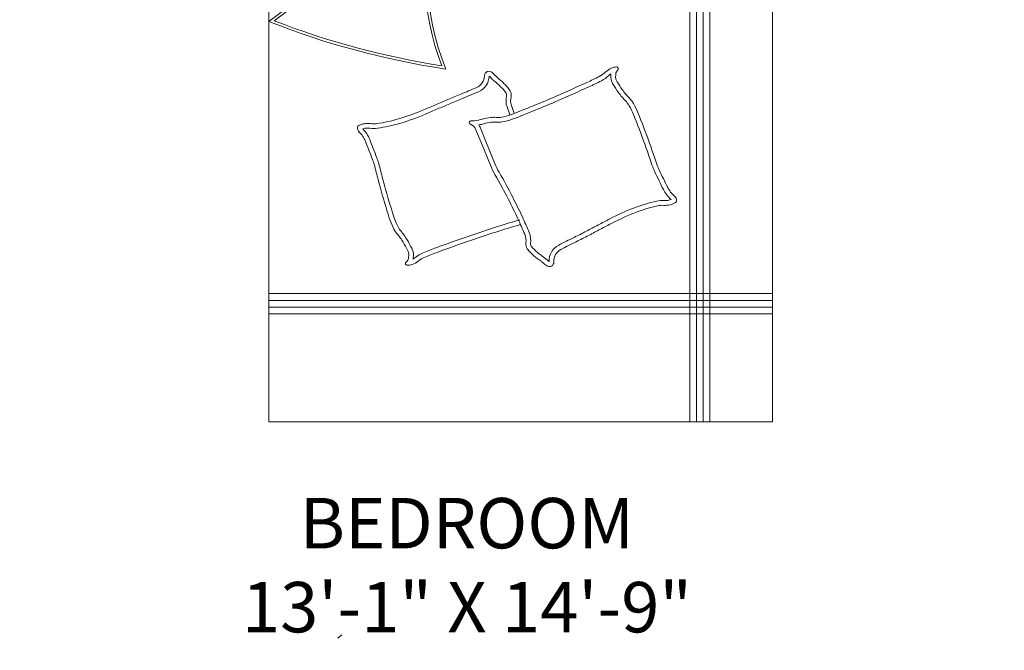
# Model space of a CAD drawing. Units: inches. Extents: x -466983 to 1020, y 324 to 318697.
# Tile 44 of 97: x 491 to 609, y 898 to 973. Entities that reach past the tile are written whole.
import ezdxf

# ---------------------------------------------------------------- set-up
doc = ezdxf.new("R2010")
doc.units = ezdxf.units.IN
doc.header["$MEASUREMENT"] = 0
for name, color, linetype, lineweight in [('A-AREA-IDEN', 7, 'Continuous', 25), ('A-FLOR-PATT', 252, 'Continuous', 13), ('A-FURN', 8, 'Continuous', 18)]:
    doc.layers.add(name, color=color, linetype=linetype, lineweight=lineweight)
doc.styles.get("Standard").update_dxf_attribs({"font": 'arial.ttf'})

# ---------------------------------------------------------------- blocks, each defined once
blk = doc.blocks.new('A$C05F852CF')
for p, q in [((0, 3.0548), (0, 2.6659)), ((0.0306, 3.0783), (0.4692, 3.0783)), ((0.4692, 3.0783), (2.0768, 3.0783)), ((0.52, 3.0783), (0.52, 1.0783)), ((2.02, 3.0783), (2.02, 1.0783)), ((2.0768, 3.0783), (2.5066, 3.0783)), ((0.5, 3.0423), (0.5, 2.6496)), ((0.52, 3.0283), (2.02, 3.0283)), ((2.04, 3.05), (2.04, 2.6642)), ((2.54, 2.6547), (2.54, 3.0393)), ((0.2418, 2.9702), (0.2418, 3.0002)), ((0.5609, 3.0045), (0.5953, 2.9829)), ((0.5609, 3.0045), (0.6121, 2.9725)), ((1.2427, 2.9995), (1.1927, 2.9682)), ((2.2982, 2.9702), (2.2982, 3.0002)), ((0.6121, 2.9725), (0.6546, 2.9682)), ((1.1927, 2.9682), (1.1672, 2.9661)), ((0.1349, 2.8634), (0.1049, 2.8634)), ((0.3487, 2.8634), (0.3787, 2.8634)), ((2.1913, 2.8634), (2.1613, 2.8634)), ((2.4051, 2.8634), (2.4351, 2.8634)), ((0.2418, 2.7265), (0.2418, 2.7565)), ((2.2982, 2.7265), (2.2982, 2.7565)), ((0.5711, 2.6712), (0.6015, 2.7135)), ((0.6015, 2.7135), (0.6164, 2.7178)), ((1.1864, 2.7072), (1.1588, 2.7242)), ((1.2397, 2.6852), (1.1864, 2.7072)), ((1.0379, 2.6608), (0.52, 2.2697)), ((2.02, 2.6608), (1.0379, 2.6608)), ((1.7737, 2.6608), (1.7737, 1.0783)), ((1.7937, 2.6608), (1.7937, 1.0783)), ((1.8137, 2.6608), (1.8137, 1.0783)), ((1.8337, 2.6608), (1.8337, 1.0783)), ((0.0322, 2.6283), (0.4826, 2.6283)), ((2.0707, 2.6283), (2.5056, 2.6283)), ((0.52, 1.4597), (2.02, 1.4597)), ((0.52, 1.4397), (2.02, 1.4397)), ((0.52, 1.4197), (2.02, 1.4197)), ((0.52, 1.3997), (2.02, 1.3997)), ((0.52, 1.0783), (2.02, 1.0783)), ((0.726, 0.4346), (0.7377, 0.4444))]:
    blk.add_line(p, q)
for points in [[(1.3405, 2.9829), (1.306, 3.0045), (1.3573, 2.9725), (1.3998, 2.9682)], [(1.9879, 2.9995), (1.9379, 2.9682), (1.9124, 2.9661)], [(1.3162, 2.6712), (1.3467, 2.7135), (1.3616, 2.7178)], [(1.9848, 2.6852), (1.9315, 2.7072), (1.9039, 2.7242)]]:
    blk.add_lwpolyline(points)
for points in [[(1.0353, 2.1379, -0.173032), (1.022, 2.6388), (0.536, 2.2719, 0.053888)], [(1.7081, 1.7759, 0.101392), (1.7282, 1.7501, -0.223768), (1.7345, 1.736, -0.25558), (1.7315, 1.7308, -0.081563), (1.7151, 1.724, -0.071805), (1.6967, 1.7225, 0.069985), (1.6778, 1.7209, 0.03546), (1.6148, 1.7021, 0.029432), (1.5425, 1.6697, 0.001554), (1.5078, 1.6515, -0.00152), (1.4724, 1.6329, -0.004735), (1.4356, 1.6142, 0.00382), (1.3901, 1.5911, 0.296001), (1.3692, 1.5546, -0.649774), (1.3468, 1.5431, -0.02319), (1.3416, 1.5477, 0.0288), (1.3374, 1.5514, 0.005727), (1.3298, 1.557, -0.004358), (1.3198, 1.5645, -0.027528), (1.3001, 1.5812, -0.046214), (1.29, 1.5928, -0.194121), (1.2856, 1.6105, 0.133719), (1.2823, 1.6363, 0.011505), (1.2622, 1.682, 0.008882), (1.2338, 1.7401, 0.012426), (1.1937, 1.8139, -0.033612), (1.1801, 1.8418), (1.1552, 1.9026), (1.1361, 1.9495, 0.224341), (1.1204, 1.9638, -0.722772), (1.1202, 1.9734, -0.103513), (1.1242, 1.9739, 0.053465), (1.132, 1.9742, 0.030109), (1.1569, 1.9792, -0.031436), (1.1808, 1.984, -0.05324), (1.1971, 1.9844, 0.05518), (1.2128, 1.9849, 0.056271), (1.2402, 1.992, 0.0108), (1.3759, 2.0475, 0.00456), (1.4675, 2.0883, 0.01125), (1.5041, 2.106, 0.069394), (1.5235, 2.1196, -0.079756), (1.5405, 2.1311, -0.106399), (1.5562, 2.1345, -0.328642), (1.5608, 2.1312, -0.299547), (1.5587, 2.124, 0.189917), (1.5536, 2.1141, 0.033518), (1.5531, 2.1029, 0.075627), (1.554, 2.0981, 0.053489), (1.5579, 2.0898, 0.017838), (1.5727, 2.0672, 0.038394), (1.5932, 2.0425, -0.059529), (1.6058, 2.026, -0.035943), (1.6193, 1.9987, -0.011245), (1.6541, 1.9079, -0.006203), (1.6684, 1.8661, 0.010783), (1.6769, 1.8422, 0.019485), (1.6828, 1.8283, 0.005062)], [(1.6953, 1.7695, 0.098587), (1.7181, 1.7399, -0.040378), (1.7118, 1.7379, -0.071805), (1.6975, 1.7367, 0.069985), (1.6747, 1.7349, 0.03546), (1.6097, 1.7154, 0.029432), (1.5359, 1.6824, 0.001554), (1.5012, 1.6641, -0.00152), (1.4658, 1.6456, -0.004735), (1.4293, 1.627, 0.00382), (1.3835, 1.6038, 0.289814), (1.3549, 1.555, -0.018279), (1.3515, 1.5579, 0.0288), (1.3461, 1.5627, 0.005727), (1.3382, 1.5686, -0.004358), (1.3285, 1.5758, -0.027528), (1.31, 1.5916, -0.046214), (1.3016, 1.6012, -0.194121), (1.2997, 1.6085, 0.133719), (1.2955, 1.6417, 0.011505), (1.2752, 1.6881, 0.008882), (1.2465, 1.7466, 0.012426), (1.2061, 1.821, -0.033612), (1.1933, 1.8472), (1.1684, 1.908), (1.1493, 1.9549, 0.051417), (1.1455, 1.962, 0.017208), (1.1606, 1.9654, -0.031436), (1.1827, 1.9698, -0.05324), (1.196, 1.9702, 0.05518), (1.2149, 1.9708, 0.056271), (1.2453, 1.9787, 0.0108), (1.3816, 2.0344, 0.00456), (1.4734, 2.0753, 0.01125), (1.5106, 2.0933, 0.069394), (1.5332, 2.1091, -0.038161), (1.5392, 2.114, 0.029361), (1.5389, 2.1025, 0.075627), (1.5405, 2.0934, 0.053489), (1.5457, 2.0824, 0.017838), (1.5611, 2.0589, 0.038394), (1.583, 2.0326, -0.059529), (1.5935, 2.0187, -0.035943), (1.6061, 1.9933, -0.011245), (1.6406, 1.9031, -0.006203), (1.6549, 1.8617, 0.010783), (1.6635, 1.8371, 0.019485), (1.6699, 1.8222, 0.005062)]]:
    blk.add_lwpolyline(points, format="xyb", close=True)
for points in [[(1.27, 1.665, 0.025626), (1.2575, 1.662, 0.0108), (1.1179, 1.617, 0.00456), (1.0234, 1.5834, 0.01125), (0.9856, 1.5685, 0.069394), (0.9653, 1.5565, -0.079756), (0.9474, 1.5464, -0.106399), (0.9315, 1.5441, -0.328642), (0.9272, 1.5478, -0.299547), (0.9298, 1.5548, 0.189917), (0.9357, 1.5643, 0.033518), (0.9369, 1.5754, 0.075627), (0.9364, 1.5803, 0.053489), (0.9332, 1.5888, 0.017838), (0.9202, 1.6125, 0.038394), (0.9016, 1.6387, -0.059529), (0.8903, 1.6561, -0.035943), (0.8789, 1.6844, -0.011245), (0.8512, 1.7776, -0.006203), (0.8402, 1.8203, 0.010783), (0.8336, 1.8448, 0.019485), (0.8287, 1.8592, 0.005062), (0.8076, 1.9133, 0.101392), (0.7895, 1.9406, -0.223768), (0.7843, 1.9551, -0.25558), (0.7876, 1.9601, -0.081563), (0.8046, 1.9656, -0.071805), (0.823, 1.9657, 0.069985), (0.842, 1.9658, 0.03546), (0.9062, 1.9798, 0.029432), (0.9807, 2.0065, 0.001554), (1.0167, 2.022, -0.00152), (1.0535, 2.0378, -0.004735), (1.0916, 2.0536, 0.00382), (1.1388, 2.0731, 0.296001), (1.1624, 2.108, -0.649774), (1.1856, 2.1178, -0.02319), (1.1904, 2.1128, 0.0288), (1.1944, 2.1088, 0.005727), (1.2015, 2.1025, -0.004358), (1.2108, 2.0944, -0.027528), (1.2292, 2.0762, -0.046214), (1.2384, 2.0638, -0.194121), (1.2414, 2.0458, 0.133719), (1.2427, 2.0199, 0.005779), (1.2507, 1.9961)], [(1.2674, 1.6787, 0.025626), (1.2535, 1.6753, 0.0108), (1.1134, 1.6301, 0.00456), (1.0187, 1.5964, 0.01125), (0.9802, 1.5813, 0.069394), (0.9566, 1.5673, -0.042175), (0.9495, 1.5626, 0.031457), (0.9508, 1.5747, 0.075627), (0.9499, 1.5838, 0.053489), (0.9456, 1.595, 0.017838), (0.9321, 1.6196, 0.038394), (0.9123, 1.6476, -0.059529), (0.9028, 1.6622, -0.035943), (0.8922, 1.6886, -0.011245), (0.8646, 1.7812, -0.006203), (0.8536, 1.8236, 0.010783), (0.8469, 1.8487, 0.019485), (0.8417, 1.8641, 0.005062), (0.8204, 1.9185, 0.100237), (0.7996, 1.9501, -0.044209), (0.8066, 1.9519, -0.071805), (0.8211, 1.952, 0.069985), (0.8439, 1.9521, 0.03546), (0.9101, 1.9665, 0.029432), (0.9862, 1.9937, 0.001554), (1.0222, 2.0093, -0.00152), (1.0589, 2.025, -0.004735), (1.0968, 2.0408, 0.00382), (1.1442, 2.0604, 0.294287), (1.1763, 2.1074, -0.02184), (1.18, 2.1036, 0.0288), (1.1851, 2.0984, 0.005727), (1.1924, 2.092, -0.004358), (1.2016, 2.084, -0.027528), (1.2189, 2.0669, -0.046214), (1.2266, 2.0566, -0.194121), (1.2279, 2.0488, 0.133719), (1.2295, 2.0156, 0.005779), (1.2376, 1.9915, 0.005779)]]:
    blk.add_lwpolyline(points, format="xyb")
for centre, radius in [((0.2418, 2.8634), 0.1369), ((2.2982, 2.8634), 0.1369), ((0.2418, 2.8634), 0.1069), ((2.2982, 2.8634), 0.1069)]:
    blk.add_circle(centre, radius)
for centre, radius, start, end in [((1.7308, 2.407), 0.7379, 159.8846, 202.2194), ((1.4058, 4.5145), 2.4132, 248.4641, 261.4655)]:
    blk.add_arc(centre, radius, start, end)
for points in [[(0, 3.0548), (0, 3.0677), (0.0177, 3.0783), (0.0306, 3.0783)], [(0.5, 3.0423), (0.5, 3.0581), (0.485, 3.0783), (0.4692, 3.0783)], [(2.04, 3.05), (2.04, 3.0655), (2.0613, 3.0783), (2.0768, 3.0783)], [(2.5066, 3.0783), (2.5237, 3.0783), (2.54, 3.0564), (2.54, 3.0393)], [(0.0322, 2.6283), (0.0157, 2.6283), (0, 2.6494), (0, 2.6659)], [(0.5, 2.6496), (0.5, 2.6405), (0.4918, 2.6283), (0.4826, 2.6283)], [(2.04, 2.6642), (2.04, 2.6485), (2.055, 2.6283), (2.0707, 2.6283)], [(2.5056, 2.6283), (2.5201, 2.6283), (2.54, 2.6403), (2.54, 2.6547)]]:
    blk.add_open_spline(points, degree=3)
for points, knots in [([(0.5609, 3.0045), (0.565, 2.9818), (0.5836, 2.9366), (0.5776, 2.889), (0.5689, 2.8351), (0.5832, 2.7709), (0.5808, 2.7088), (0.5744, 2.6927), (0.5693, 2.6651), (0.5803, 2.6793), (0.5989, 2.6876), (0.7172, 2.6598), (0.8681, 2.7029), (1.0484, 2.6781), (1.0324, 2.6731), (1.1431, 2.7116), (1.202, 2.6757), (1.2459, 2.6867), (1.2222, 2.695), (1.2359, 2.7251), (1.2468, 2.781), (1.2288, 2.8492), (1.2515, 2.925), (1.2279, 2.9609), (1.2471, 3.0058), (1.2098, 2.9902), (1.1177, 3.0095), (0.956, 3.0159), (0.9532, 2.9758), (0.7999, 3.021), (0.7569, 3.0151), (0.5986, 2.9869), (0.561, 3.0049)], [16.816032, 16.816032, 16.816032, 16.816032, 79.038845, 88.513895, 147.565266, 227.196862, 259.685448, 283.955301, 296.511304, 302.432558, 320.230942, 354.322559, 575.279549, 734.72356, 845.740421, 943.033103, 1029.533967, 1032.845074, 1043.313584, 1065.311534, 1104.921835, 1208.53002, 1248.510714, 1303.102727, 1321.01326, 1329.647833, 1389.371624, 1571.817644, 1750.274161, 1823.189073, 1967.937033, 2020.912329, 2020.912329, 2020.912329, 2020.912329]), ([(1.306, 3.0045), (1.3102, 2.9818), (1.3287, 2.9366), (1.3228, 2.889), (1.314, 2.8351), (1.3284, 2.7709), (1.3259, 2.7088), (1.3196, 2.6927), (1.3144, 2.6651), (1.3254, 2.6793), (1.3441, 2.6876), (1.4624, 2.6598), (1.6132, 2.7029), (1.6436, 2.6781), (1.7775, 2.6731), (1.8882, 2.7116), (1.9472, 2.6757), (1.9911, 2.6867), (1.9673, 2.695), (1.981, 2.7251), (1.992, 2.781), (1.974, 2.8492), (1.9967, 2.925), (1.9731, 2.9609), (1.9922, 3.0058), (1.9549, 2.9902), (1.8628, 3.0095), (1.7011, 3.0159), (1.5483, 2.9758), (1.5451, 3.021), (1.5021, 3.0151), (1.3437, 2.9869), (1.3062, 3.0049)], [16.816032, 16.816032, 16.816032, 16.816032, 79.038845, 88.513895, 147.565266, 227.196862, 259.685448, 283.955301, 296.511304, 302.432558, 320.230942, 354.322559, 575.279549, 734.72356, 845.740421, 943.033103, 1029.533967, 1032.845074, 1043.313584, 1065.311534, 1104.921835, 1208.53002, 1248.510714, 1303.102727, 1321.01326, 1329.647833, 1389.371624, 1571.817644, 1750.274161, 1823.189073, 1967.937033, 2020.912329, 2020.912329, 2020.912329, 2020.912329]), ([(1.186, 2.943), (1.1557, 2.9456), (1.1387, 2.9502), (1.0976, 2.9551), (1.0776, 2.9567), (1.0342, 2.9582), (1.0123, 2.957), (0.991, 2.9533), (0.9902, 2.9517), (0.962, 2.9403), (0.9371, 2.935), (0.8851, 2.9413), (0.8522, 2.9513), (0.8033, 2.9629), (0.7938, 2.964), (0.755, 2.9608), (0.7319, 2.9572), (0.6794, 2.9481), (0.658, 2.9434), (0.631, 2.9418)], [1364.380335, 1364.380335, 1364.380335, 1364.380335, 1423.60231, 1423.60231, 1482.824284, 1482.824284, 1566.205036, 1566.205036, 1649.585789, 1649.585789, 1732.966542, 1732.966542, 1816.347295, 1816.347295, 1899.728048, 1899.728048, 1960.499853, 1960.499853, 1990.525565, 1990.525565, 1990.525565, 1990.525565]), ([(0.631, 2.9418), (0.6332, 2.9288), (0.633, 2.9104), (0.6308, 2.893), (0.6298, 2.8865), (0.628, 2.8726), (0.6273, 2.866), (0.6257, 2.8474), (0.6257, 2.8375), (0.629, 2.8013), (0.6345, 2.7696), (0.6337, 2.7333)], [67.285362, 67.285362, 67.285362, 67.285362, 87.399558, 87.399558, 107.513754, 107.513754, 127.62795, 127.62795, 167.856341, 167.856341, 238.127268, 238.127268, 238.127268, 238.127268]), ([(1.1845, 2.7412), (1.189, 2.7552), (1.1894, 2.765), (1.1874, 2.7998), (1.1843, 2.8219), (1.1844, 2.8664), (1.1882, 2.8901), (1.192, 2.9105), (1.1922, 2.9144), (1.1921, 2.9158), (1.1908, 2.9212), (1.1875, 2.9351), (1.1867, 2.9388), (1.186, 2.943)], [1072.516901, 1072.516901, 1072.516901, 1072.516901, 1129.100964, 1129.100964, 1185.685027, 1185.685027, 1226.035089, 1226.035089, 1249.281274, 1249.281274, 1272.52746, 1272.52746, 1279.689275, 1279.689275, 1279.689275, 1279.689275]), ([(1.3759, 2.942), (1.3781, 2.929), (1.378, 2.9106), (1.3757, 2.893), (1.3748, 2.8866), (1.373, 2.8727), (1.3722, 2.8661), (1.3706, 2.8475), (1.3707, 2.8375), (1.3739, 2.8012), (1.3795, 2.7694), (1.3787, 2.7331)], [67.156228, 67.156228, 67.156228, 67.156228, 87.297212, 87.297212, 107.438196, 107.438196, 127.57918, 127.57918, 167.861148, 167.861148, 238.25357, 238.25357, 238.25357, 238.25357]), ([(1.5104, 2.9621), (1.4964, 2.9606), (1.4732, 2.9568), (1.4226, 2.948), (1.4017, 2.9435), (1.3759, 2.942)], [1904.3965, 1904.3965, 1904.3965, 1904.3965, 1961.927876, 1961.927876, 1990.619445, 1990.619445, 1990.619445, 1990.619445]), ([(1.9314, 2.9432), (1.8997, 2.9459), (1.8822, 2.9507), (1.8387, 2.9557), (1.8168, 2.9572), (1.7515, 2.9587), (1.7088, 2.9551), (1.6403, 2.9447), (1.6154, 2.9402), (1.5795, 2.937), (1.5675, 2.9361), (1.5394, 2.9412), (1.5201, 2.9507), (1.5104, 2.9621)], [1364.265661, 1364.265661, 1364.265661, 1364.265661, 1426.240795, 1426.240795, 1488.215928, 1488.215928, 1612.166195, 1612.166195, 1689.92864, 1689.92864, 1733.064362, 1733.064362, 1768.978829, 1768.978829, 1768.978829, 1768.978829]), ([(1.9299, 2.7409), (1.9344, 2.755), (1.9348, 2.7648), (1.9328, 2.7996), (1.9297, 2.8217), (1.9298, 2.8662), (1.9336, 2.8899), (1.9374, 2.9105), (1.9376, 2.9144), (1.9375, 2.9159), (1.9362, 2.9214), (1.9329, 2.9353), (1.9321, 2.939), (1.9314, 2.9432)], [1072.238498, 1072.238498, 1072.238498, 1072.238498, 1128.864869, 1128.864869, 1185.491239, 1185.491239, 1225.989553, 1225.989553, 1249.326401, 1249.326401, 1272.66325, 1272.66325, 1279.788508, 1279.788508, 1279.788508, 1279.788508]), ([(0.6337, 2.7333), (0.6515, 2.7301), (0.6627, 2.7284), (0.6898, 2.7263), (0.7032, 2.726), (0.7436, 2.727), (0.7707, 2.73), (0.8409, 2.7383), (0.8881, 2.7432), (0.9755, 2.7406), (1.0125, 2.7357), (1.0356, 2.7309), (1.0369, 2.7307), (1.0381, 2.7304)], [345.4047, 345.4047, 345.4047, 345.4047, 383.386056, 383.386056, 421.367413, 421.367413, 497.330126, 497.330126, 611.561469, 611.561469, 725.792813, 725.792813, 732.434768, 732.434768, 732.434768, 732.434768]), ([(1.0381, 2.7304), (1.0497, 2.7345), (1.0742, 2.7435), (1.1251, 2.7504), (1.1528, 2.749), (1.1769, 2.7432), (1.1809, 2.7421), (1.1845, 2.7412)], [843.64503, 843.64503, 843.64503, 843.64503, 911.27572, 911.27572, 959.088062, 959.088062, 969.47998, 969.47998, 969.47998, 969.47998]), ([(1.3787, 2.7331), (1.3984, 2.7296), (1.4106, 2.7278), (1.4401, 2.7258), (1.4545, 2.7258), (1.4962, 2.7276), (1.5219, 2.7313), (1.5767, 2.7399), (1.6067, 2.7436), (1.6527, 2.7371), (1.662, 2.7326), (1.7084, 2.7282), (1.7364, 2.7276), (1.7849, 2.734), (1.8076, 2.7406), (1.8563, 2.7489), (1.8812, 2.7508), (1.914, 2.7451), (1.9226, 2.7428), (1.9299, 2.7409)], [345.267918, 345.267918, 345.267918, 345.267918, 387.167414, 387.167414, 429.06691, 429.06691, 512.865903, 512.865903, 629.317545, 629.317545, 745.769188, 745.769188, 834.622813, 834.622813, 901.414409, 901.414409, 948.921878, 948.921878, 969.679511, 969.679511, 969.679511, 969.679511])]:
    blk.add_open_spline(points, degree=3, knots=knots)
for p in [(0.2366, 2.8475), (2.3034, 2.8475), (0.2309, 2.8244), (2.02, 1.0783), (2.02, 1.0783)]:
    blk.add_point(p)

msp = doc.modelspace()

# ---------------------------------------------------------------- hatches: boundary and pattern name
at = {"layer": 'A-FLOR-PATT', "transparency": 33554572}
h = msp.add_hatch(dxfattribs=at)
h.set_pattern_fill('ANSI37', color=256, scale=30)
h.set_pattern_definition([(45, (-1212.4137, -290.035), (-2.6516504, 2.6516504), []), (135, (-1212.4137, -290.035), (-2.6516504, -2.6516504), [])])
h.paths.add_polyline_path([(901.81, 1075.94), (900.61, 1075.94), (900.61, 1065.39), (899.39, 1065.39), (898.09, 1065.39), (892.84, 1058.71, -0.258377), (892.19, 1058.35), (879.98, 1058.35, -0.20177), (879.44, 1058.58), (874.08, 1065.39), (872.78, 1065.39), (871.56, 1065.39), (871.56, 1075.94), (813.81, 1075.94), (813.81, 1044.79), (832.39, 1044.79, -0.394795), (848.66, 1028.54), (848.66, 1009.94), (901.81, 1009.94), (901.81, 1015.94), (901.31, 1015.94), (871.31, 1015.94), (871.31, 1017.25), (871.33, 1017.25, -0.401453), (901.31, 1045.94), (901.81, 1045.94)])
edge = h.paths.add_edge_path(flags=16)
edge.add_line((847.77, 1068.95), (847.77, 1073.71))
edge.add_arc((849.23, 1073.71), 1.45, 90, 180, ccw=False)
edge.add_line((849.23, 1075.16), (864.49, 1075.16))
edge.add_arc((864.49, 1073.71), 1.45, 0, 90, ccw=False)
edge.add_line((865.95, 1073.71), (865.95, 1069))
edge.add_arc((832.64, 1068.98), 33.3, -20.6123, 0.0472, ccw=False)
edge.add_ellipse((856.86, 1058.48), major_axis=(0, 10.21), ratio=0.685919, start_angle=100.0088, end_angle=259.9912, ccw=False)
edge.add_arc((881.07, 1068.98), 33.3, 180.0472, 200.6123, ccw=False)
h.paths.add_polyline_path([(853.15, 1066.48), (853.15, 1066.45), (853.15, 1066.45, 0.433107), (852.92, 1066.68), (852.92, 1066.45), (853.15, 1066.45), (853.15, 1066.48), (853.09, 1066.61, 0.697939), (852.7, 1066.45), (852.7, 1066.45), (852.7, 1066.48), (852.92, 1067), (852.92, 1066.68, -0.396254)], flags=0)
h.paths.add_polyline_path([(861.02, 1066.48), (861.02, 1066.45), (861.02, 1066.45, 0.416404), (860.8, 1066.68), (860.8, 1066.45), (861.02, 1066.45), (861.02, 1066.48), (860.97, 1066.61, 0.713344), (860.57, 1066.45), (860.57, 1066.45), (860.57, 1066.48), (860.8, 1067), (860.8, 1066.68, -0.379973)], flags=0)
edge = h.paths.add_edge_path(flags=0)
edge.add_spline(control_points=[(861.13, 1065.79), (861.47, 1065.25), (861.61, 1065.02), (861.98, 1064.37), (862.19, 1063.94), (862.56, 1063.04), (862.72, 1062.56), (862.99, 1061.58), (863.09, 1061.07), (863.25, 1060.03), (863.29, 1059.5), (863.33, 1058.44), (863.32, 1057.91), (863.24, 1056.85), (863.17, 1056.33), (862.97, 1055.31), (862.84, 1054.81), (862.54, 1053.85), (862.36, 1053.39), (861.95, 1052.52), (861.73, 1052.12), (861.23, 1051.36), (860.97, 1051.02), (860.4, 1050.39), (860.11, 1050.12), (859.49, 1049.65), (859.18, 1049.45), (858.53, 1049.13), (858.2, 1049.01), (857.53, 1048.85), (857.2, 1048.81), (856.52, 1048.81), (856.19, 1048.85), (855.52, 1049.01), (855.19, 1049.13), (854.54, 1049.45), (854.23, 1049.64), (853.61, 1050.12), (853.32, 1050.39), (852.75, 1051.01), (852.49, 1051.36), (852, 1052.11), (851.77, 1052.52), (851.36, 1053.39), (851.18, 1053.85), (850.88, 1054.81), (850.75, 1055.31), (850.55, 1056.33), (850.48, 1056.85), (850.4, 1057.9), (850.39, 1058.44), (850.43, 1059.5), (850.47, 1060.03), (850.63, 1061.07), (850.73, 1061.58), (851, 1062.56), (851.16, 1063.04), (851.53, 1063.94), (851.73, 1064.37), (852.11, 1065.02), (852.25, 1065.25), (852.61, 1065.73)], knot_values=[3.915332, 3.915332, 3.915332, 3.915332, 4.013468, 4.013468, 4.175532, 4.175532, 4.337596, 4.337596, 4.49966, 4.49966, 4.661724, 4.661724, 4.823788, 4.823788, 4.985852, 4.985852, 5.147916, 5.147916, 5.30998, 5.30998, 5.472044, 5.472044, 5.634109, 5.634109, 5.796173, 5.796173, 5.958237, 5.958237, 6.120301, 6.120301, 6.282365, 6.282365, 6.444429, 6.444429, 6.606493, 6.606493, 6.768557, 6.768557, 6.930621, 6.930621, 7.092685, 7.092685, 7.254749, 7.254749, 7.416813, 7.416813, 7.578878, 7.578878, 7.740942, 7.740942, 7.903006, 7.903006, 8.06507, 8.06507, 8.227134, 8.227134, 8.389198, 8.389198, 8.551262, 8.551262, 8.65037, 8.65037, 8.65037, 8.65037], degree=3, periodic=0)
edge.add_line((852.64, 1065.79), (861.13, 1065.79))
edge = h.paths.add_edge_path(flags=0)
edge.add_ellipse((856.85, 1057.74), major_axis=(0, 7.79), ratio=0.687861, start_angle=0, end_angle=360)
h.paths.add_polyline_path([(848.86, 1069.39), (848.86, 1073.96, -0.414214), (849.95, 1075.05), (863.77, 1075.05, -0.414214), (864.86, 1073.96), (864.86, 1069.39, -0.388936), (864.52, 1069.03, -0.043561), (849.2, 1069.03, -0.388936)], flags=0)
h.paths.add_polyline_path([(853.1, 1068.11, -1), (852.68, 1068.11, -1)], flags=0)
edge = h.paths.add_edge_path(flags=0)
edge.add_ellipse((856.86, 1057.34), major_axis=(0, 2.21), ratio=0.657164, start_angle=0, end_angle=360)
h.paths.add_polyline_path([(861.04, 1068.11, -1), (860.62, 1068.11, -1)], flags=0)
edge = h.paths.add_edge_path()
edge.add_line((573.95, 1057.34), (573.95, 1075.94))
edge.add_line((573.95, 1075.94), (558.73, 1075.94))
edge.add_line((558.73, 1075.94), (558.73, 1065.39))
edge.add_line((558.73, 1065.39), (557.51, 1065.39))
edge.add_line((557.51, 1065.39), (556.21, 1065.39))
edge.add_line((556.21, 1065.39), (550.95, 1058.71))
edge.add_arc((550.3, 1059.12), 0.765, 270, 327.9483, ccw=False)
edge.add_line((550.3, 1058.35), (538.1, 1058.35))
edge.add_arc((538.1, 1059.12), 0.765, 224.3704, 270, ccw=False)
edge.add_line((537.55, 1058.58), (532.2, 1065.39))
edge.add_line((532.2, 1065.39), (530.9, 1065.39))
edge.add_line((530.9, 1065.39), (529.67, 1065.39))
edge.add_line((529.67, 1065.39), (529.67, 1075.94))
edge.add_line((529.67, 1075.94), (520.81, 1075.94))
edge.add_line((520.81, 1075.94), (520.81, 1045.94))
edge.add_line((520.81, 1045.94), (521.31, 1045.94))
edge.add_arc((521.31, 1015.94), 30, 2.5075, 90, ccw=False)
edge.add_line((551.28, 1017.25), (551.31, 1017.25))
edge.add_line((551.31, 1017.25), (551.31, 1015.94))
edge.add_line((551.31, 1015.94), (520.81, 1015.94))
edge.add_line((520.81, 1015.94), (520.81, 1009.94))
edge.add_line((520.81, 1009.94), (559.19, 1010.4))
edge.add_arc((559.19, 1011.86), 1.45, 180, 270, ccw=False)
edge.add_line((557.74, 1011.86), (557.74, 1016.56))
edge.add_arc((591.04, 1016.59), 33.3, 159.3877, 180.0472, ccw=False)
edge.add_ellipse((566.82, 1027.08), major_axis=(0, 10.21), ratio=0.685919, start_angle=280.0088, end_angle=439.9912, ccw=False)
edge.add_arc((542.61, 1016.59), 33.3, 0.0472, 20.6123, ccw=False)
edge.add_line((575.91, 1016.62), (575.91, 1011.86))
edge.add_arc((574.46, 1011.86), 1.45, -90, 0, ccw=False)
edge.add_line((574.46, 1010.4), (608.81, 1009.94))
edge.add_line((608.81, 1009.94), (608.81, 1041.09))
edge.add_line((608.81, 1041.09), (590.22, 1041.09))
edge.add_arc((590.78, 1057.91), 16.83, 181.9277, 268.1032, ccw=False)
edge = h.paths.add_edge_path()
edge.add_ellipse((494.24, 583.62), major_axis=(0, 10.21), ratio=0.685919, start_angle=280.0088, end_angle=439.9912, ccw=False)
edge.add_arc((470.03, 573.12), 33.3, 0.0472, 20.6123, ccw=False)
edge.add_line((503.33, 573.15), (503.33, 568.39))
edge.add_arc((501.88, 568.39), 1.45, -90, 0, ccw=False)
edge.add_line((501.88, 566.94), (539.81, 566.94))
edge.add_line((539.81, 566.94), (539.81, 572.94))
edge.add_line((539.81, 572.94), (539.31, 572.94))
edge.add_line((539.31, 572.94), (509.31, 572.94))
edge.add_line((509.31, 572.94), (509.31, 574.25))
edge.add_line((509.31, 574.25), (509.33, 574.25))
edge.add_arc((539.31, 572.94), 30, 90, 177.4925, ccw=False)
edge.add_line((539.31, 602.94), (539.81, 602.94))
edge.add_line((539.81, 602.94), (539.81, 626.94))
edge.add_line((539.81, 626.94), (531.77, 626.94))
edge.add_line((531.77, 626.94), (531.77, 616.39))
edge.add_line((531.77, 616.39), (530.55, 616.39))
edge.add_line((530.55, 616.39), (529.25, 616.39))
edge.add_line((529.25, 616.39), (523.71, 609.35))
edge.add_line((523.71, 609.35), (510.78, 609.35))
edge.add_line((510.78, 609.35), (505.24, 616.39))
edge.add_line((505.24, 616.39), (503.94, 616.39))
edge.add_line((503.94, 616.39), (502.72, 616.39))
edge.add_line((502.72, 616.39), (502.72, 626.94))
edge.add_line((502.72, 626.94), (481.7, 626.94))
edge.add_line((481.7, 626.94), (481.7, 611))
edge.add_arc((467.27, 611.47), 14.44, 271.9277, 358.1032, ccw=False)
edge.add_line((467.76, 597.05), (451.81, 597.05))
edge.add_line((451.81, 597.05), (451.81, 584.4))
edge.add_line((451.81, 584.4), (451.81, 566.94))
edge.add_line((451.81, 566.94), (486.61, 566.94))
edge.add_arc((486.61, 568.39), 1.45, 180, 270, ccw=False)
edge.add_line((485.16, 568.39), (485.16, 573.1))
edge.add_arc((518.46, 573.12), 33.3, 159.3877, 180.0472, ccw=False)
h.paths.add_polyline_path([(836.26, 1020.73), (879.89, 1020.73), (879.89, 1039.39), (836.26, 1039.39)], flags=25)
h.paths.add_polyline_path([(549.99, 1036.75), (593.61, 1036.75), (593.61, 1055.41), (549.99, 1055.41)], flags=24)
h.paths.add_polyline_path([(475.12, 595.6), (518.75, 595.6), (518.75, 614.25), (475.12, 614.25)], flags=24)

# ---------------------------------------------------------------- block references
at = {"layer": 'A-FURN', "xscale": 40, "yscale": 40, "zscale": 40}
msp.add_blockref('A$C05F852CF', (500.37, 881.77), dxfattribs=at)

# ---------------------------------------------------------------- texts
at = {"layer": 'A-AREA-IDEN', "insert": (430, 915.83), "char_height": 6, "attachment_point": 1}
msp.add_mtext_dynamic_manual_height_columns('\\pxqc;{\\fArial|b1|i0|c0|p34;BEDROOM\\P13\'-1" X 14\'-9"}', width=229.5583, gutter_width=1, heights=[0], dxfattribs=at)

doc.saveas('drawing.dxf')
